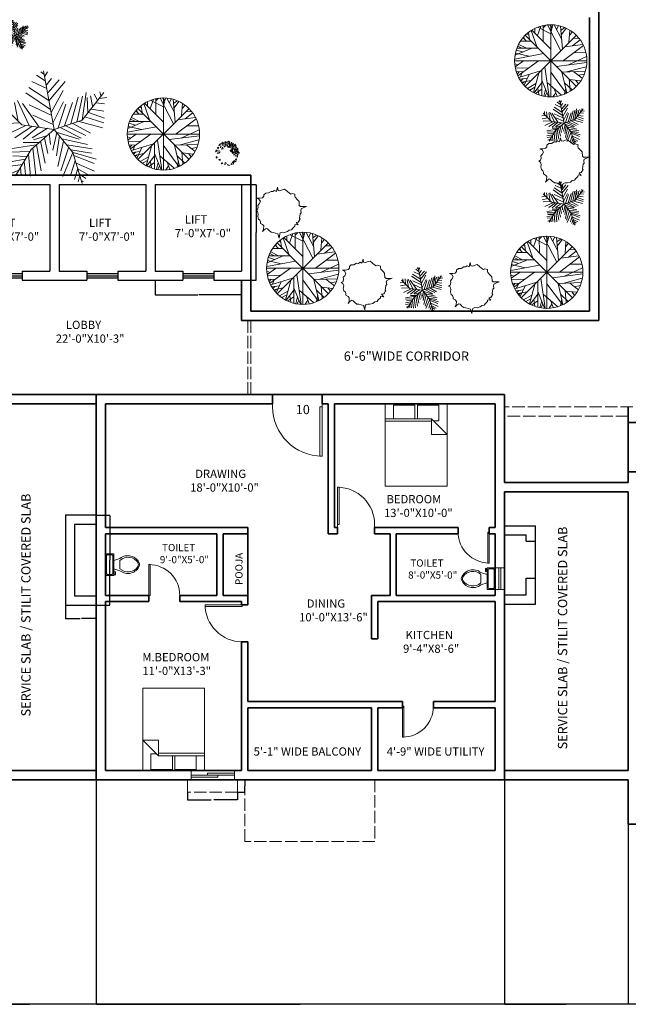
# Model space of a CAD drawing. Units: inches. Extents: x -69 to 2453, y 4803 to 7122.
# Tile 5 of 9: x 1203 to 1794, y 4803 to 5759. Entities that reach past the tile are written whole.
import ezdxf

# ---------------------------------------------------------------- set-up
doc = ezdxf.new("R2010")
doc.units = ezdxf.units.IN
doc.linetypes.add('ACAD_ISO02W100', pattern=[15, 12, -3])
for name, color, linetype, lineweight in [('A-ANNO-DIMS', 2, 'Continuous', 18), ('A-ANNO-IDEN', 2, 'Continuous', 18), ('A-AREA-IDEN', 7, 'Continuous', 18), ('A-DOOR', 3, 'Continuous', 18), ('A-FLOR-EVTR', 4, 'Continuous', 25), ('A-FLOR-FIXT', 9, 'Continuous', 18), ('A-FLOR-OVHD', 8, 'ACAD_ISO02W100', 13), ('A-FURN', 8, 'Continuous', 18), ('A-GLAZ', 244, 'Continuous', 18), ('A-WALL', 7, 'Continuous', 35), ('A-WALL-SRVC', 7, 'Continuous', 30), ('L-PLNT', 94, 'Continuous', 13)]:
    doc.layers.add(name, color=color, linetype=linetype, lineweight=lineweight)
doc.styles.get("Standard").update_dxf_attribs({"font": 'arial.ttf'})
doc.dimstyles.get("Standard").update_dxf_attribs({"dimtxt": 0.18, "dimasz": 0.18, "dimexe": 0.18, "dimexo": 0.0625, "dimgap": 0.09, "dimtad": 0, "dimtih": 1, "dimtoh": 1, "dimdec": 4, "dimzin": 0, "dimdsep": 46, "dimtxsty": 'Standard', "dimcen": 0.09, "dimadec": 0, "dimazin": 0, "dimtfac": 1, "dimtdec": 4, "dimtofl": 0, "dimtmove": 0, "dimatfit": 3, "dimfxl": 1, "dimtolj": 1, "dimtzin": 0, "dimarcsym": 0})

# ---------------------------------------------------------------- blocks, each defined once
blk = doc.blocks.new('*U6')
for p, q in [((-40, 0), (-40, 6)), ((0, 0), (0, 6))]:
    blk.add_line(p, q)
blk.add_lwpolyline([(0, 0), (0, -40), (-1.75, -40), (-1.75, 0)], close=True)
blk.add_arc((0, 0), 40, 180, 270)
blk = doc.blocks.new('*U17')
for p, q in [((0, 0), (0, 6)), ((40, 0), (40, 6))]:
    blk.add_line(p, q)
blk.add_lwpolyline([(0, 0), (0, -40), (1.75, -40), (1.75, 0)], close=True)
blk.add_arc((0, 0), 40, 270, 0)
blk = doc.blocks.new('*U5')
for p, q in [((0, 0), (0, -6)), ((40, 0), (40, -6))]:
    blk.add_line(p, q)
blk.add_lwpolyline([(0, 0), (0, 40), (1.75, 40), (1.75, 0)], close=True)
blk.add_arc((0, 0), 40, 0, 90)
blk = doc.blocks.new('*U3')
for p, q in [((0, 0), (0, 6)), ((40, 0), (40, 6))]:
    blk.add_line(p, q)
blk.add_lwpolyline([(0, 0), (0, -40), (1.75, -40), (1.75, 0)], close=True)
blk.add_arc((0, 0), 40, 270, 360)
blk = doc.blocks.new('*U22')
for p, q in [((0, 0), (0, -6)), ((40, 0), (40, -6))]:
    blk.add_line(p, q)
blk.add_lwpolyline([(0, 0), (0, 40), (1.75, 40), (1.75, 0)], close=True)
blk.add_arc((0, 0), 40, 0, 90)
blk = doc.blocks.new('*U29')
blk.add_lwpolyline([(-4.577, 66.508), (-7.629, 55.26), (-12.588, 57.705), (-17.165, 54.771), (-22.124, 55.26), (-29.372, 50.859), (-36.619, 50.37), (-41.578, 45.968), (-41.578, 42.056), (-45.393, 37.655), (-52.259, 36.677), (-60.651, 36.677), (-54.929, 33.743), (-51.115, 27.385), (-54.548, 21.028), (-58.362, 17.116), (-57.599, 11.248), (-58.744, 5.379), (-63.703, 2.445), (-59.125, 0), (-56.837, -6.846), (-58.362, -13.204), (-56.455, -20.539), (-52.259, -23.473), (-51.115, -27.386), (-51.115, -32.276), (-45.011, -35.21), (-41.96, -39.122), (-42.723, -47.925), (-45.393, -54.282), (-40.434, -49.392), (-35.475, -45.969), (-31.66, -46.947), (-27.083, -51.837), (-21.361, -56.238), (-16.021, -56.727), (-3.433, -60.151), (0, -71.887), (1.526, -60.151), (3.052, -58.194), (8.392, -56.238), (14.114, -56.727), (22.506, -54.282), (27.465, -50.37), (33.95, -49.392), (37.002, -44.991), (42.723, -39.611), (43.105, -35.699), (45.012, -34.721), (51.878, -36.188), (46.157, -29.342), (51.878, -28.364), (53.785, -25.919), (56.074, -21.517), (57.6, -20.539), (55.693, -18.094), (57.219, -5.868), (59.889, -2.934), (58.744, 3.423), (60.27, 7.824), (67.137, 11.248), (74.766, 14.182), (67.899, 13.693), (58.363, 13.693), (54.93, 16.627), (54.167, 27.874), (50.353, 32.276), (43.868, 39.122), (42.723, 42.545), (43.105, 47.436), (35.476, 49.881), (31.661, 47.925), (27.084, 50.859), (14.496, 61.128), (9.155, 59.661), (2.289, 56.727), (-3.051, 57.705)], close=True)
blk = doc.blocks.new('*U25')
for p, q in [((-8.737, 47.138), (-17.069, 52.711)), ((-10.186, 53.64), (-13.084, 55.962)), ((0, 0), (-10.5, 57)), ((-9.099, 51.782), (-6.563, 55.962)), ((-7.65, 43.423), (-2.578, 49.46)), ((-5.839, 35.992), (4.667, 48.067)), ((-5.114, 28.097), (-24.676, 40.636)), ((-7.288, 39.707), (-21.778, 46.673)), ((-5.114, 27.632), (10.463, 46.673)), ((-48.585, 21.131), (-49.309, 29.026)), ((-3.665, 19.273), (-27.574, 35.527)), ((-2.941, 16.486), (8.652, 37.85)), ((16.259, 5.805), (23.142, 31.348)), ((22.055, 7.198), (27.489, 32.277)), ((27, 9), (48, 36)), ((27.127, 9.056), (31.112, 35.992)), ((31.836, 30.883), (32.561, 16.486)), ((35.096, 32.741), (37.27, 22.524)), ((38.719, 34.134), (41.979, 28.561)), ((43.791, 29.954), (51.036, 30.883)), ((44.153, 36.456), (45.239, 32.741)), ((-47.498, 19.737), (-55.83, 18.344)), ((-31.5, 4.5), (-52.5, 25.5)), ((-43.513, 28.561), (-42.427, 15.558)), ((-38.442, 26.239), (-34.819, 7.663)), ((-35.544, 28.097), (-24.314, 3.947)), ((-14.533, 2.09), (-30.834, 25.31)), ((-24.314, 23.917), (-2.941, 13.7)), ((-1.129, 6.734), (9.014, 26.704)), ((3.942, 1.625), (11.187, 24.381)), ((10.101, 3.483), (17.708, 26.239)), ((36.183, 19.737), (48.137, 17.88)), ((40.53, 25.775), (48.862, 24.846)), ((-40.615, 13.7), (-55.105, 10.913)), ((-20.691, 13.7), (-1.129, 4.876)), ((29.662, 12.307), (48.137, 6.269)), ((33.285, 16.486), (48.862, 10.913)), ((-33.37, 6.269), (-52.207, 5.34)), ((-28.299, 3.483), (-47.86, -5.805)), ((-21.416, 3.018), (-38.079, -8.128)), ((0, 0), (-31.5, 4.5)), ((-15.982, 2.09), (-30.11, -9.521)), ((0, 0), (-22.5, -19.5)), ((-6.563, 1.161), (-21.416, -8.128)), ((0, 0), (27, 9)), ((0, 0), (18, -22.5)), ((6.478, 1.625), (26.04, -8.592)), ((11.187, 3.483), (30.749, -5.805)), ((18.07, 5.805), (35.096, -3.483)), ((24.229, 7.663), (46.688, 1.625)), ((-6.563, -5.805), (-19.967, -9.985)), ((-9.461, -8.592), (-6.201, -23.453)), ((-4.752, -3.483), (-3.665, -14.629)), ((2.493, -3.019), (-1.491, -20.202)), ((1.769, -2.555), (24.229, -9.521)), ((5.029, -6.27), (2.131, -25.775)), ((7.565, -9.056), (32.198, -14.629)), ((-17.431, -15.094), (-42.789, -18.809)), ((-15.257, -12.772), (-30.11, -12.772)), ((-20.691, -18.345), (-17.793, -44.352)), ((-17.069, -15.094), (-12.721, -40.172)), ((-13.446, -11.378), (-8.737, -32.741)), ((9.014, -11.378), (3.58, -35.992)), ((14.085, -16.951), (6.478, -40.172)), ((12.274, -15.094), (36.907, -18.809)), ((-24.314, -21.596), (-42.427, -22.06)), ((-26.849, -26.24), (-40.253, -25.775)), ((-22.5, -19.5), (-37.5, -45)), ((-25.038, -23.918), (-22.865, -45.281)), ((18.07, -22.524), (8.289, -45.745)), ((16.259, -19.738), (36.183, -22.989)), ((18, -22.5), (27, -52.5)), ((18.433, -22.524), (40.53, -29.026)), ((19.157, -25.311), (38.719, -33.206)), ((-28.299, -29.026), (-42.789, -31.348)), ((-30.834, -34.135), (-42.427, -35.528)), ((-32.646, -36.921), (-31.921, -44.352)), ((-29.023, -30.884), (-27.936, -43.887)), ((20.244, -30.419), (15.897, -44.816)), ((22.78, -37.85), (19.519, -48.532)), ((21.331, -32.741), (39.081, -40.636)), ((-34.457, -39.708), (-40.978, -42.494)), ((22.78, -38.314), (34.372, -44.816)), ((24.591, -45.745), (23.142, -50.854)), ((24.591, -43.423), (30.749, -47.603)), ((26.764, -49.925), (28.213, -50.854))]:
    blk.add_line(p, q)
blk = doc.blocks.new('*U28')
for p, q in [((-32.6092, 50.4264), (-23.2782, 23.5674)), ((-31.2008, 51.1035), (-0.2149, 20.1818)), ((-26.4472, 46.5894), (-26.2712, 53.8116)), ((-22.0458, 42.0753), (-16.5881, 57.6486)), ((-21.1656, 55.8436), (-0.0388, 45.0094)), ((-12.5388, 54.9406), (-7.9613, 59.4546)), ((-12.3627, 32.1443), (-12.5388, 58.7776)), ((-5.3205, 59.6806), (16.5105, 16.7963)), ((2.426, 54.9406), (-1.4472, 59.9056)), ((0, 59.9996), (0, -60)), ((0.4894, 48.6208), (3.6584, 59.6806)), ((18.2711, 35.5298), (5.419, 59.6806)), ((9.8203, 51.5549), (12.8133, 58.5516)), ((19.6795, 19.5047), (16.3344, 57.6486)), ((17.0387, 51.1035), (23.2006, 55.1666)), ((17.7429, 43.6552), (25.4894, 54.2636)), ((31.6513, 50.8778), (30.2429, 30.5643)), ((-49.8627, 32.8214), (-32.7853, 32.8214)), ((-45.8134, 38.2383), (-40.5318, 33.0471)), ((-43.8768, 36.4326), (-44.405, 40.2696)), ((42, 42), (-42, -42)), ((42, -42), (-42, 42)), ((-40.1797, 44.558), (-36.4825, 43.2038)), ((-37.0107, 47.0408), (-35.25, 35.5298)), ((31.1232, 42.5267), (35.8767, 48.1693)), ((36.2288, 25.1474), (48.9049, 35.0784)), ((37.1091, 37.1098), (46.6161, 37.5612)), ((-32.2571, 20.6333), (-59.1937, 9.348)), ((-57.081, 17.9248), (-47.0458, 14.7649)), ((-56.0247, 20.859), (-20.8134, 20.859)), ((-54.7923, 24.4702), (-47.75, 21.0847)), ((-53.2078, 27.4044), (-40.1797, 20.859)), ((54.3626, 25.3731), (20.9119, 0.3198)), ((23.3767, 23.3417), (53.3063, 27.4044)), ((-59.7219, 2.8025), (-12.0106, 12.0565)), ((-58.6656, 12.7336), (-35.9543, 7.5424)), ((-54.6162, -24.7335), (-20.2853, 0.0941)), ((29.3626, -6.6771), (59.4682, 7.091)), ((38.5175, 13.4107), (58.2359, 13.6364)), ((-60, 0), (60, 0)), ((-59.7219, -4.8714), (-54.2641, -6.6771)), ((-45.2853, -0.1316), (-59.0177, -10.0627)), ((-58.4895, -12.3197), (-36.4825, -11.6426)), ((-14.8275, -15.0282), (-14.6515, -57.6865)), ((-10.074, -10.0627), (-2.5036, -59.7178)), ((9.2922, -9.1598), (59.6443, -2.8401)), ((26.3697, -18.4138), (58.9401, -9.8369)), ((-57.081, -18.4138), (-45.2853, -17.9624)), ((-52.6797, -18.188), (-55.4966, -22.0251)), ((-53.2078, -27.442), (-16.7641, -16.6081)), ((-38.9472, -29.0219), (-51.4472, -30.6018)), ((-47.2219, -19.3166), (-50.2148, -26.3135)), ((-46.5177, -30.1504), (-49.5106, -33.536)), ((-32.4331, -32.4075), (-48.1021, -35.5674)), ((-35.9543, -22.4765), (-44.0529, -40.5329)), ((-19.9331, -20.2194), (-28.5599, -52.721)), ((-14.6515, -32.1818), (-3.912, -59.4922)), ((-0.0388, -19.0909), (25.8415, -53.8495)), ((18.6232, -18.6394), (26.7218, -53.3981)), ((18.7992, -18.6394), (57.3556, -17.2853)), ((30.419, -30.1504), (32.3556, -50.0125)), ((31.4753, -31.279), (49.6091, -33.3103)), ((38.1654, -18.188), (52.426, -29.0219)), ((41.5105, -32.6332), (46.088, -38.0501)), ((45.9119, -24.0564), (55.595, -22.2508)), ((-43.7008, -34.6645), (-46.6937, -37.373)), ((-24.6867, -37.8244), (-38.7712, -45.7241)), ((-26.2712, -43.9185), (-34.7219, -48.6583)), ((-14.6515, -36.2445), (-27.6797, -52.9467)), ((-14.6515, -47.3041), (-25.0388, -54.3009)), ((-21.5177, -45.4984), (-19.9331, -56.1065)), ((-8.4895, -47.5298), (-11.4825, -58.5893)), ((-6.2008, -36.2445), (17.919, -57.0094)), ((5.9471, -46.6269), (10.5246, -58.5893)), ((22.8485, -36.4702), (35.3485, -48.4326)), ((24.7852, -44.8213), (23.0246, -54.978)), ((-6.3768, -52.721), (-9.3698, -58.815)), ((8.4119, -53.1724), (3.8344, -59.4922))]:
    blk.add_line(p, q)
blk.add_circle((0, 0), 60)
blk = doc.blocks.new('*U27')
for points in [[(-5.78, 9.75), (-7.54, 9.23), (-8.01, 7.5), (-6.26, 8.45)], [(-4.43, 11.05), (-5.18, 10.36), (-3.96, 9.49), (-2.07, 10.36)], [(-2, 11.66), (-1.6, 10.62), (-0.52, 10.1), (-0.18, 10.62), (-0.79, 10.96)], [(1.24, 12), (0.56, 11.31), (0.76, 10.01), (2.52, 11.05)], [(2.59, 9.93), (1.84, 9.75), (1.64, 9.23), (2.32, 9.41)], [(4.14, 11.14), (3.6, 10.01), (4, 9.23), (5.22, 8.71), (6.3, 9.41), (5.08, 10.19), (4.61, 10.01)], [(-11.32, 1.79), (-9.83, 2.31), (-9.63, 3.44), (-10.44, 3.52)], [(-8.21, 0.41), (-9.43, 0.32), (-9.83, 0.84)], [(-8.14, 6.03), (-9.36, 5.95), (-9.02, 4.73)], [(-8.21, 3.09), (-8.48, 2.31), (-7.87, 2.57)], [(-7, 1.79), (-7.94, 1.53), (-7.47, 0.49)], [(-5.78, 6.81), (-6.66, 6.21), (-6.52, 5.69)], [(-4.57, 6.38), (-5.45, 4.47), (-3.89, 4.82)], [(-4.84, 8.63), (-3.83, 7.85), (-4.03, 8.97)], [(-2.88, 7.5), (-3.15, 6.64), (-2.27, 6.72)], [(-1.94, 9.49), (-2.48, 8.97), (-2.27, 8.54), (-1.8, 9.06)], [(0.02, 9.06), (-1.33, 8.54), (-1.73, 7.16), (0.29, 7.76)], [(0.76, 7.16), (0.09, 6.46), (1.1, 5.95)], [(1.37, 8.54), (3.13, 8.8), (3.8, 7.85), (1.91, 7.76)], [(1.71, 6.29), (1.71, 7.07), (2.65, 7.5), (2.11, 6.9)], [(2.52, 6.81), (2.52, 5.86), (4.41, 5.17), (4.61, 6.72)], [(3.53, 1.88), (2.86, 3.52), (3.8, 3.52)], [(4.41, 4.56), (4.27, 3.7), (5.49, 3.26)], [(4.27, 2.74), (5.29, 2.66), (4.41, 1.27)], [(4.61, 8.28), (4.54, 7.76), (4.95, 7.59), (4.95, 8.28)], [(5.83, 1.53), (5.02, 0.41), (5.49, -0.02), (6.5, 0.41)], [(5.49, 5.51), (5.42, 4.82), (6.16, 5.08)], [(6.43, 7.94), (5.49, 7.68), (5.56, 6.21), (6.5, 6.64)], [(7.51, 1.71), (6.91, 1.27), (6.23, 2.14)], [(8.12, 4.99), (7.11, 4.65), (6.5, 4.13), (7.38, 3.09), (8.12, 3.52), (7.65, 3.87)], [(7.45, 9.32), (7.11, 7.94), (8.52, 7.94)], [(7.85, 6.81), (7.18, 6.21), (9, 5.51), (9.33, 6.38)], [(8.12, 0.75), (7.51, 0.15), (8.93, -0.28), (9.13, 0.49)], [(8.19, 2.57), (7.92, 2.05), (8.66, 1.53)], [(8.73, 4.73), (8.19, 4.56), (8.39, 3.87), (8.59, 4.04)], [(10.28, 5.17), (9.2, 4.04), (9, 2.31), (10.48, 0.49), (11.76, 0.41), (10.35, 2.48), (9.33, 2.4), (10.28, 2.83)], [(-10.03, -2.71), (-10.64, -3.31), (-10.44, -4.44), (-9.9, -3.49)], [(-8.28, -5.73), (-6.79, -5.3), (-7, -6.51)], [(-4.84, -8.85), (-4.43, -9.45), (-5.99, -9.8)], [(-2.34, -9.2), (-1.26, -8.5), (-0.99, -9.54)], [(4.07, -9.45), (3.53, -9.97), (4.07, -10.58), (4.61, -9.89)], [(5.29, -7.98), (4.61, -8.16), (5.02, -8.94)], [(6.03, -9.45), (5.42, -9.97), (6.16, -10.15)], [(6.1, -8.94), (6.16, -7.21), (6.91, -6.69), (7.24, -7.38)], [(7.78, -0.8), (6.43, -1.5), (6.43, -0.72)], [(8.32, -1.75), (7.98, -2.53), (7.58, -2.1)], [(8.05, -8.07), (8.59, -7.12), (7.92, -7.55)], [(9.33, -5.13), (8.46, -6.25), (7.98, -5.22)], [(9.33, -1.75), (9.54, -3.74), (10.14, -2.53)], [(10.08, -0.63), (9.74, -1.32), (10.48, -0.89)], [(-2.54, -10.06), (-3.02, -10.23), (-1.8, -10.67)], [(0.22, -10.58), (0.83, -11.27), (2.59, -11.36)]]:
    blk.add_lwpolyline(points, close=True)
blk = doc.blocks.new('Bed - Queen')
for p, q in [((0, -80.00003), (0, 0)), ((0, 0), (59.99999, 0)), ((59.99999, 0), (59.99999, -80.00003)), ((7.99999, -1.2), (28.79998, -1.2)), ((7.99999, -14.4), (7.99999, -1.2)), ((28.79998, -1.2), (28.79998, -14.4)), ((31.19999, -1.2), (51.99999, -1.2)), ((31.19999, -14.4), (31.19999, -1.2)), ((51.99999, -1.2), (51.99999, -16.4)), ((0, -14.4), (44.8, -14.4)), ((44.8, -16.8), (0, -16.8)), ((59.99999, -29.6), (44.8, -14.4)), ((44.8, -14.4), (44.8, -29.6)), ((51.99999, -16.4), (46.79936, -16.4)), ((44.8, -29.6), (59.99999, -29.6)), ((59.99999, -80.00003), (0, -80.00003))]:
    blk.add_line(p, q)
blk = doc.blocks.new('*U33')
for p, q in [((-10, -8.5), (-8, -8.5)), ((-10, -9.5), (-10, -8.5)), ((-7, -9.5), (-10, -9.5)), ((-8, -8.5), (-8, -8)), ((-7, -8), (-7, -9.5)), ((-4, -8), (-6, -14)), ((4, -8), (6, -14)), ((9.5, -6), (9.5, -2)), ((4, -14), (-4, -14))]:
    blk.add_line(p, q)
blk.add_lwpolyline([(10.5, -8), (10.5, 0), (-10.5, 0), (-10.5, -8)], close=True)
for points in [[(-9.5, -2), (-9.5, -6)], [(8.5, -1), (-8.5, -1)], [(-8.5, -7), (8.5, -7)]]:
    blk.add_lwpolyline(points)
for centre, radius, start, end in [((-8.62, -1.88), 0.884, 81.8699, 188.1301), ((-8.62, -6.12), 0.884, 171.8699, 278.1301), ((8.62, -1.88), 0.884, 351.8699, 98.1301), ((8.62, -6.12), 0.884, 261.8699, 8.1301), ((3.52, -21.58), 12.17, 141.46911, 247.97143), ((4.2, -21.82), 11.33, 136.36773, 238.94682), ((-3.52, -21.58), 12.17, 292.02843, 38.53071), ((-4.2, -21.82), 11.33, 301.05301, 43.63209), ((0, -27.88), 4, 245.73182, 294.26817), ((0, -29), 4, 254.86053, 285.13947)]:
    blk.add_arc(centre, radius, start, end)
blk = doc.blocks.new('WINDOW-VENT-21IN')
for p, q in [((0, 5.5), (21, 5.5)), ((0, 3.5), (21, 3.5))]:
    blk.add_line(p, q)
blk.add_lwpolyline([(0, 9), (21, 9), (21, 0), (0, 0)], close=True)
blk = doc.blocks.new('WINDOW-SLIDING-42IN')
for p, q in [((2.5, 42), (2.5, 16)), ((4.5, 42), (4.5, 0)), ((4.5, 26), (6.5, 26)), ((6.5, 26), (6.5, 0)), ((4.5, 16), (2.5, 16))]:
    blk.add_line(p, q)
blk.add_lwpolyline([(0, 42), (9, 42), (9, 0), (0, 0)], close=True)
blk = doc.blocks.new('SUNSHADE-48IN')
for p, q in [((0, 0), (0, 12)), ((48.4, 12), (48.4, 0)), ((48.4, 0), (0, 0))]:
    blk.add_line(p, q)
blk = doc.blocks.new('SERVICE-BAY-87IN')
for p, q in [((30, 87.24), (0, 87.24)), ((0, 87.24), (0, 0)), ((30, 78.24), (9, 78.24)), ((9, 78.24), (9, 9)), ((0, 0), (30, 0)), ((9, 9), (30, 9))]:
    blk.add_line(p, q)
blk = doc.blocks.new('LIFT-PASSENGER-84IN')
for p, q in [((0, 93), (84, 93)), ((0, 93), (0, 9)), ((84, 93), (84, 9)), ((0, 9), (27, 9)), ((27, 9), (27, 0)), ((27, 6.5), (57, 6.5)), ((27, 4.5), (57, 4.5)), ((27, 2.5), (57, 2.5)), ((57, 9), (57, 0)), ((57, 9), (84, 9))]:
    blk.add_line(p, q)
blk = doc.blocks.new('*D55')
at = {"layer": 'A-ANNO-DIMS', "color": 0, "lineweight": -2, "transparency": 16777216}
for p, q in [((1365.97, 5008.65), (1365.97, 5001.28)), ((1366.15, 5001.46), (1388.91, 5001.46)), ((1414.19, 5001.46), (1391.43, 5001.46)), ((1414.37, 5008.65), (1414.37, 5001.28))]:
    blk.add_line(p, q, dxfattribs=at)
at = {"layer": 'A-ANNO-DIMS', "color": 0, "transparency": 16777216}
for points in [[(1366.15, 5001.49), (1366.15, 5001.43), (1365.97, 5001.46)], [(1414.19, 5001.49), (1414.19, 5001.43), (1414.37, 5001.46)]]:
    blk.add_solid(points, dxfattribs=at)
at = {"layer": 'Defpoints', "color": 0, "transparency": 16777216}
for p in [(1365.97, 5008.72), (1414.37, 5008.72), (1414.37, 5001.46)]:
    blk.add_point(p, dxfattribs=at)
at = {"layer": 'A-ANNO-DIMS', "color": 0, "transparency": 16777216, "insert": (1390.17, 5001.46), "char_height": 0.18, "attachment_point": 5}
blk.add_mtext('\\A1;SUNSHADE 48 TYP.', dxfattribs=at)
blk = doc.blocks.new('*D56')
at = {"layer": 'A-ANNO-DIMS', "color": 0, "lineweight": -2, "transparency": 16777216}
for p, q in [((1414.43, 5020.72), (1421.81, 5020.72)), ((1421.63, 5020.54), (1421.63, 5014.9)), ((1421.63, 5008.9), (1421.63, 5014.53)), ((1414.43, 5008.72), (1421.81, 5008.72))]:
    blk.add_line(p, q, dxfattribs=at)
at = {"layer": 'A-ANNO-DIMS', "color": 0, "transparency": 16777216}
for points in [[(1421.6, 5020.54), (1421.66, 5020.54), (1421.63, 5020.72)], [(1421.6, 5008.9), (1421.66, 5008.9), (1421.63, 5008.72)]]:
    blk.add_solid(points, dxfattribs=at)
at = {"layer": 'Defpoints', "color": 0, "transparency": 16777216}
for p in [(1414.37, 5020.72), (1421.63, 5020.72), (1414.37, 5008.72)]:
    blk.add_point(p, dxfattribs=at)
at = {"layer": 'A-ANNO-DIMS', "color": 0, "transparency": 16777216, "insert": (1421.63, 5014.72), "char_height": 0.18, "attachment_point": 5}
blk.add_mtext('\\A1;12 TYP.', dxfattribs=at)
blk = doc.blocks.new('*D71')
at = {"layer": 'A-ANNO-DIMS', "color": 0, "lineweight": -2, "transparency": 16777216}
for p, q in [((1418.57, 5598.72), (1432.64, 5598.72)), ((1432.46, 5598.54), (1432.46, 5552.4)), ((1432.46, 5505.9), (1432.46, 5552.03)), ((1418.57, 5505.72), (1432.64, 5505.72))]:
    blk.add_line(p, q, dxfattribs=at)
at = {"layer": 'A-ANNO-DIMS', "color": 0, "transparency": 16777216}
for points in [[(1432.43, 5598.54), (1432.49, 5598.54), (1432.46, 5598.72)], [(1432.43, 5505.9), (1432.49, 5505.9), (1432.46, 5505.72)]]:
    blk.add_solid(points, dxfattribs=at)
at = {"layer": 'Defpoints', "color": 0, "transparency": 16777216}
for p in [(1418.51, 5598.72), (1432.46, 5598.72), (1418.51, 5505.72)]:
    blk.add_point(p, dxfattribs=at)
at = {"layer": 'A-ANNO-DIMS', "color": 0, "transparency": 16777216, "insert": (1432.46, 5552.22), "char_height": 0.18, "attachment_point": 5}
blk.add_mtext('\\A1;PASSENGER LIFT 93 TYP.', dxfattribs=at)
blk = doc.blocks.new('*D72')
at = {"layer": 'A-ANNO-DIMS', "color": 0, "lineweight": -2, "transparency": 16777216}
for p, q in [((1334.51, 5505.65), (1334.51, 5491.59)), ((1418.51, 5505.65), (1418.51, 5491.59)), ((1334.69, 5491.77), (1375.98, 5491.77)), ((1418.33, 5491.77), (1377.04, 5491.77))]:
    blk.add_line(p, q, dxfattribs=at)
at = {"layer": 'A-ANNO-DIMS', "color": 0, "transparency": 16777216}
for points in [[(1334.69, 5491.8), (1334.69, 5491.74), (1334.51, 5491.77)], [(1418.33, 5491.8), (1418.33, 5491.74), (1418.51, 5491.77)]]:
    blk.add_solid(points, dxfattribs=at)
at = {"layer": 'Defpoints', "color": 0, "transparency": 16777216}
for p in [(1334.51, 5505.72), (1418.51, 5505.72), (1418.51, 5491.77)]:
    blk.add_point(p, dxfattribs=at)
at = {"layer": 'A-ANNO-DIMS', "color": 0, "transparency": 16777216, "insert": (1376.51, 5491.77), "char_height": 0.18, "attachment_point": 5}
blk.add_mtext('\\A1;84 TYP.', dxfattribs=at)
blk = doc.blocks.new('*D77')
at = {"layer": 'A-ANNO-DIMS', "color": 0, "lineweight": -2, "transparency": 16777216}
for p, q in [((1277.57, 5277.65), (1290.78, 5277.65)), ((1290.6, 5277.47), (1290.6, 5234.21)), ((1290.6, 5190.59), (1290.6, 5233.84)), ((1277.57, 5190.41), (1290.78, 5190.41))]:
    blk.add_line(p, q, dxfattribs=at)
at = {"layer": 'A-ANNO-DIMS', "color": 0, "transparency": 16777216}
for points in [[(1290.57, 5277.47), (1290.63, 5277.47), (1290.6, 5277.65)], [(1290.57, 5190.59), (1290.63, 5190.59), (1290.6, 5190.41)]]:
    blk.add_solid(points, dxfattribs=at)
at = {"layer": 'Defpoints', "color": 0, "transparency": 16777216}
for p in [(1277.51, 5277.65), (1290.6, 5277.65), (1277.51, 5190.41)]:
    blk.add_point(p, dxfattribs=at)
at = {"layer": 'A-ANNO-DIMS', "color": 0, "transparency": 16777216, "insert": (1290.6, 5234.03), "char_height": 0.18, "attachment_point": 5}
blk.add_mtext('\\A1;SERVICE BAY 87 TYP.', dxfattribs=at)
blk = doc.blocks.new('*D78')
at = {"layer": 'A-ANNO-DIMS', "color": 0, "lineweight": -2, "transparency": 16777216}
for p, q in [((1247.51, 5190.34), (1247.51, 5177.14)), ((1277.51, 5190.34), (1277.51, 5177.14)), ((1247.69, 5177.32), (1261.98, 5177.32)), ((1277.33, 5177.32), (1263.04, 5177.32))]:
    blk.add_line(p, q, dxfattribs=at)
at = {"layer": 'A-ANNO-DIMS', "color": 0, "transparency": 16777216}
for points in [[(1247.69, 5177.35), (1247.69, 5177.29), (1247.51, 5177.32)], [(1277.33, 5177.35), (1277.33, 5177.29), (1277.51, 5177.32)]]:
    blk.add_solid(points, dxfattribs=at)
at = {"layer": 'Defpoints', "color": 0, "transparency": 16777216}
for p in [(1247.51, 5190.41), (1277.51, 5190.41), (1277.51, 5177.32)]:
    blk.add_point(p, dxfattribs=at)
at = {"layer": 'A-ANNO-DIMS', "color": 0, "transparency": 16777216, "insert": (1262.51, 5177.32), "char_height": 0.18, "attachment_point": 5}
blk.add_mtext('\\A1;30 TYP.', dxfattribs=at)
blk = doc.blocks.new('*D84')
at = {"layer": 'A-ANNO-DIMS', "color": 0, "lineweight": -2, "transparency": 16777216}
for p, q in [((1148.51, 5020.65), (1148.51, 4802.79)), ((1277.51, 5020.65), (1277.51, 4802.79)), ((1148.69, 4802.97), (1212.73, 4802.97)), ((1277.33, 4802.97), (1213.29, 4802.97))]:
    blk.add_line(p, q, dxfattribs=at)
at = {"layer": 'A-ANNO-DIMS', "color": 0, "transparency": 16777216}
for points in [[(1148.69, 4803), (1148.69, 4802.94), (1148.51, 4802.97)], [(1277.33, 4803), (1277.33, 4802.94), (1277.51, 4802.97)]]:
    blk.add_solid(points, dxfattribs=at)
at = {"layer": 'Defpoints', "color": 0, "transparency": 16777216}
for p in [(1148.51, 5020.72), (1277.51, 5020.72), (1277.51, 4802.97)]:
    blk.add_point(p, dxfattribs=at)
at = {"layer": 'A-ANNO-DIMS', "color": 0, "transparency": 16777216, "insert": (1213.01, 4802.97), "char_height": 0.18, "attachment_point": 5}
blk.add_mtext('\\A1;129', dxfattribs=at)
blk = doc.blocks.new('*D85')
at = {"layer": 'A-ANNO-DIMS', "color": 0, "lineweight": -2, "transparency": 16777216}
for p, q in [((1277.51, 5020.65), (1277.51, 4802.79)), ((1673.51, 5020.65), (1673.51, 4802.79)), ((1277.69, 4802.97), (1475.22, 4802.97)), ((1673.33, 4802.97), (1475.8, 4802.97))]:
    blk.add_line(p, q, dxfattribs=at)
at = {"layer": 'A-ANNO-DIMS', "color": 0, "transparency": 16777216}
for points in [[(1277.69, 4803), (1277.69, 4802.94), (1277.51, 4802.97)], [(1673.33, 4803), (1673.33, 4802.94), (1673.51, 4802.97)]]:
    blk.add_solid(points, dxfattribs=at)
at = {"layer": 'Defpoints', "color": 0, "transparency": 16777216}
for p in [(1277.51, 5020.72), (1673.51, 5020.72), (1673.51, 4802.97)]:
    blk.add_point(p, dxfattribs=at)
at = {"layer": 'A-ANNO-DIMS', "color": 0, "transparency": 16777216, "insert": (1475.51, 4802.97), "char_height": 0.18, "attachment_point": 5}
blk.add_mtext('\\A1;396', dxfattribs=at)
blk = doc.blocks.new('*D86')
at = {"layer": 'A-ANNO-DIMS', "color": 0, "lineweight": -2, "transparency": 16777216}
for p, q in [((1673.51, 5020.65), (1673.51, 4802.79)), ((1793.51, 5020.65), (1793.51, 4802.79)), ((1673.69, 4802.97), (1733.23, 4802.97)), ((1793.33, 4802.97), (1733.79, 4802.97))]:
    blk.add_line(p, q, dxfattribs=at)
at = {"layer": 'A-ANNO-DIMS', "color": 0, "transparency": 16777216}
for points in [[(1673.69, 4803), (1673.69, 4802.94), (1673.51, 4802.97)], [(1793.33, 4803), (1793.33, 4802.94), (1793.51, 4802.97)]]:
    blk.add_solid(points, dxfattribs=at)
at = {"layer": 'Defpoints', "color": 0, "transparency": 16777216}
for p in [(1673.51, 5020.72), (1793.51, 5020.72), (1793.51, 4802.97)]:
    blk.add_point(p, dxfattribs=at)
at = {"layer": 'A-ANNO-DIMS', "color": 0, "transparency": 16777216, "insert": (1733.51, 4802.97), "char_height": 0.18, "attachment_point": 5}
blk.add_mtext('\\A1;120', dxfattribs=at)
blk = doc.blocks.new('*D95')
at = {"layer": 'A-ANNO-DIMS', "color": 0, "lineweight": -2, "transparency": 16777216}
for p, q in [((96.509262, 5020.652777), (96.509262, 4802.785277)), ((2286.509262, 4977.652777), (2286.509262, 4802.785277)), ((96.689262, 4802.965277), (1191.149262, 4802.965277)), ((2286.329262, 4802.965277), (1191.869262, 4802.965277))]:
    blk.add_line(p, q, dxfattribs=at)
at = {"layer": 'A-ANNO-DIMS', "color": 0, "transparency": 16777216}
for points in [[(96.689262, 4802.995277), (96.689262, 4802.935277), (96.509262, 4802.965277)], [(2286.329262, 4802.995277), (2286.329262, 4802.935277), (2286.509262, 4802.965277)]]:
    blk.add_solid(points, dxfattribs=at)
at = {"layer": 'Defpoints', "color": 0, "transparency": 16777216}
for p in [(96.509262, 5020.715277), (2286.509262, 4977.715277), (2286.509262, 4802.965277)]:
    blk.add_point(p, dxfattribs=at)
at = {"layer": 'A-ANNO-DIMS', "color": 0, "transparency": 16777216, "insert": (1191.509262, 4802.965277), "char_height": 0.18, "attachment_point": 5}
blk.add_mtext('\\A1;2190', dxfattribs=at)
blk = doc.blocks.new('*D105')
at = {"layer": 'A-ANNO-DIMS', "color": 0, "lineweight": -2, "transparency": 16777216}
for p, q in [((66.509262, 5170.610035), (66.509262, 4802.785277)), ((2316.509262, 5140.587945), (2316.509262, 4802.785277)), ((66.689262, 4802.965277), (1191.149262, 4802.965277)), ((2316.329262, 4802.965277), (1191.869262, 4802.965277))]:
    blk.add_line(p, q, dxfattribs=at)
at = {"layer": 'A-ANNO-DIMS', "color": 0, "transparency": 16777216}
for points in [[(66.689262, 4802.995277), (66.689262, 4802.935277), (66.509262, 4802.965277)], [(2316.329262, 4802.995277), (2316.329262, 4802.935277), (2316.509262, 4802.965277)]]:
    blk.add_solid(points, dxfattribs=at)
at = {"layer": 'Defpoints', "color": 0, "transparency": 16777216}
for p in [(66.509262, 5170.672535), (2316.509262, 5140.650445), (2316.509262, 4802.965277)]:
    blk.add_point(p, dxfattribs=at)
at = {"layer": 'A-ANNO-DIMS', "color": 0, "transparency": 16777216, "insert": (1191.509262, 4802.965277), "char_height": 0.18, "attachment_point": 5}
blk.add_mtext('\\A1;2250', dxfattribs=at)

msp = doc.modelspace()

# ---------------------------------------------------------------- linework, layer by layer
at = {"layer": 'A-FLOR-EVTR'}
for p, q in [((1205.51, 5505.72), (1268.51, 5505.72)), ((1298.51, 5505.72), (1361.51, 5505.72)), ((1391.51, 5505.72), (1418.51, 5505.72))]:
    msp.add_line(p, q, dxfattribs=at)
at = {"layer": 'A-FLOR-OVHD'}
for p, q in [((1424.51, 5466.72), (1424.51, 5394.72)), ((1427.51, 5466.72), (1427.51, 5394.72)), ((1843.01, 5382.72), (1673.51, 5382.72)), ((1793.51, 5373.72), (1673.51, 5373.72)), ((1421.76, 4960.72), (1421.76, 5020.72)), ((1547.6, 5020.72), (1547.6, 4960.72)), ((1547.6, 4960.72), (1421.76, 4960.72))]:
    msp.add_line(p, q, dxfattribs=at)
at = {"layer": 'A-WALL'}
for p, q in [((1765.01, 6087.72), (1765.01, 5466.72)), ((1756.01, 5760.72), (1756.01, 5475.72)), ((857.51, 5607.72), (1427.51, 5607.72)), ((1427.51, 5607.72), (1427.51, 5475.72)), ((1418.51, 5505.72), (1418.51, 5466.72)), ((1427.51, 5475.72), (1756.01, 5475.72)), ((1418.51, 5466.72), (1765.01, 5466.72)), ((752.51, 5394.72), (1673.51, 5394.72)), ((1277.51, 5394.72), (1277.51, 5020.72)), ((1448.51, 5385.72), (1448.51, 5394.72)), ((1496.51, 5385.72), (1496.51, 5394.72)), ((1673.51, 5394.72), (1673.51, 5309.33)), ((1148.51, 5385.72), (1277.51, 5385.72)), ((1286.51, 5385.72), (1286.51, 5265.72)), ((1286.51, 5385.72), (1448.51, 5385.72)), ((1496.51, 5385.72), (1502.51, 5385.72)), ((1502.51, 5385.72), (1502.51, 5259.72)), ((1508.51, 5385.72), (1508.51, 5265.72)), ((1508.51, 5385.72), (1664.51, 5385.72)), ((1664.51, 5385.72), (1664.51, 5265.72)), ((1793.51, 5382.72), (1793.51, 5309.33)), ((1802.51, 5367.72), (1793.51, 5367.72)), ((1802.51, 5319.72), (1793.51, 5319.72)), ((1673.51, 5309.33), (1793.51, 5309.33)), ((1673.51, 5300.33), (1793.51, 5300.33)), ((1673.51, 5300.33), (1673.51, 5020.72)), ((1793.51, 5300.33), (1793.51, 5029.72)), ((1286.51, 5265.72), (1424.51, 5265.72)), ((1286.51, 5259.72), (1394.51, 5259.72)), ((1286.51, 5259.72), (1286.51, 5199.72)), ((1394.51, 5259.72), (1394.51, 5199.72)), ((1400.51, 5259.72), (1400.51, 5199.72)), ((1400.51, 5259.72), (1424.51, 5259.72)), ((1424.51, 5265.72), (1424.51, 5190.72)), ((1502.51, 5259.72), (1511.51, 5259.72)), ((1508.51, 5265.72), (1511.51, 5265.72)), ((1511.51, 5265.72), (1511.51, 5259.72)), ((1547.51, 5265.72), (1547.51, 5259.72)), ((1547.51, 5265.72), (1628.51, 5265.72)), ((1547.51, 5259.72), (1562.51, 5259.72)), ((1562.51, 5259.72), (1562.51, 5199.72)), ((1568.51, 5259.72), (1568.51, 5199.72)), ((1568.51, 5259.72), (1628.51, 5259.72)), ((1628.51, 5265.72), (1628.51, 5259.72)), ((1658.51, 5265.72), (1658.51, 5259.72)), ((1658.51, 5265.72), (1664.51, 5265.72)), ((1658.51, 5259.72), (1664.51, 5259.72)), ((1664.51, 5259.72), (1664.51, 5199.72)), ((1286.51, 5199.72), (1328.51, 5199.72)), ((1286.51, 5193.72), (1328.51, 5193.72)), ((1286.51, 5193.72), (1286.51, 5029.72)), ((1328.51, 5199.72), (1328.51, 5193.72)), ((1358.51, 5199.72), (1358.51, 5193.72)), ((1358.51, 5199.72), (1394.51, 5199.72)), ((1358.51, 5193.72), (1418.51, 5193.72)), ((1400.51, 5199.72), (1424.51, 5199.72)), ((1418.51, 5193.72), (1418.51, 5190.72)), ((1544.51, 5199.72), (1562.51, 5199.72)), ((1544.51, 5199.72), (1544.51, 5157.72)), ((1550.51, 5193.72), (1664.51, 5193.72)), ((1550.51, 5193.72), (1550.51, 5157.72)), ((1568.51, 5199.72), (1664.51, 5199.72)), ((1664.51, 5193.72), (1664.51, 5096.72)), ((1418.51, 5190.72), (1424.51, 5190.72)), ((1418.51, 5154.72), (1424.51, 5154.72)), ((1418.51, 5154.72), (1418.51, 5029.72)), ((1424.51, 5154.72), (1424.51, 5096.72)), ((1550.51, 5157.72), (1544.51, 5157.72)), ((1424.51, 5096.72), (1574.51, 5096.72)), ((1574.51, 5090.72), (1574.51, 5096.72)), ((1604.51, 5090.72), (1604.51, 5096.72)), ((1604.51, 5096.72), (1664.51, 5096.72)), ((1424.51, 5090.72), (1544.51, 5090.72)), ((1424.51, 5090.72), (1424.51, 5029.72)), ((1544.51, 5090.72), (1544.51, 5029.72)), ((1550.51, 5090.72), (1550.51, 5029.72)), ((1550.51, 5090.72), (1574.51, 5090.72)), ((1604.51, 5090.72), (1664.51, 5090.72)), ((1664.51, 5090.72), (1664.51, 5029.72)), ((1148.51, 5029.72), (1277.51, 5029.72)), ((1286.51, 5029.72), (1418.51, 5029.72)), ((1424.51, 5029.72), (1544.51, 5029.72)), ((1550.51, 5029.72), (1664.51, 5029.72)), ((1673.51, 5029.72), (1793.51, 5029.72)), ((354.66, 5020.72), (1793.51, 5020.72)), ((1793.51, 5020.72), (1793.51, 4977.72)), ((1793.51, 4977.72), (2286.51, 4977.72))]:
    msp.add_line(p, q, dxfattribs=at)
at = {"layer": 'A-WALL-SRVC'}
for p, q in [((1673.51, 5267.45), (1703.51, 5267.45)), ((1703.51, 5191.38), (1703.51, 5267.45)), ((1673.51, 5258.45), (1694.51, 5258.45)), ((1694.51, 5252.38), (1694.51, 5258.45)), ((1694.51, 5252.38), (1703.51, 5252.38)), ((1694.51, 5216.38), (1703.51, 5216.38)), ((1694.51, 5200.38), (1694.51, 5216.38)), ((1673.51, 5200.38), (1694.51, 5200.38)), ((1673.51, 5191.38), (1703.51, 5191.38))]:
    msp.add_line(p, q, dxfattribs=at)

# ---------------------------------------------------------------- block references
at = {"layer": 'A-DOOR'}
for name, p, xscale, yscale, zscale in [('*U6', (1496.51, 5383.02), 1.199999999999977, 1.199999999999977, 1.199999999999977), ('*U5', (1511.51, 5268.72), 0.9, 0.9, 0.9), ('*U6', (1658.51, 5261.22), 0.7500000000000029, 0.7500000000000029, 0.7500000000000029), ('*U22', (1328.51, 5199.72), 0.7500000000000029, 0.7500000000000029, 0.7500000000000029), ('*U3', (1574.51, 5092.22), 0.7500000000000029, 0.7500000000000029, 0.7500000000000029)]:
    msp.add_blockref(name, p, dxfattribs=dict(at, xscale=xscale, yscale=yscale, zscale=zscale))
at = {"layer": 'A-DOOR', "xscale": 0.9, "yscale": 0.9, "zscale": 0.9, "rotation": 270}
msp.add_blockref('*U17', (1419.11, 5190.72), dxfattribs=at)
at = {"layer": 'A-FLOR-EVTR'}
for p in [(1148.51, 5505.72), (1241.51, 5505.72), (1334.51, 5505.72)]:
    msp.add_blockref('LIFT-PASSENGER-84IN', p, dxfattribs=at)
at = {"layer": 'A-FLOR-FIXT'}
for p, rotation in [((1286.51, 5229.72), 89.99999999999999), ((1664.51, 5216.01), 270)]:
    msp.add_blockref('*U33', p, dxfattribs=dict(at, rotation=rotation))
at = {"layer": 'A-FLOR-OVHD'}
msp.add_blockref('SUNSHADE-48IN', (1365.97, 5008.72), dxfattribs=at)
at = {"layer": 'A-FURN'}
msp.add_blockref('Bed - Queen', (1557.71, 5385.72), dxfattribs=at)
at = {"layer": 'A-FURN', "rotation": 180}
msp.add_blockref('Bed - Queen', (1382.51, 5029.72), dxfattribs=at)
at = {"layer": 'A-GLAZ'}
for name, p, rotation in [('WINDOW-VENT-21IN', (1664.51, 5226.51), 269.999999999998), ('WINDOW-SLIDING-42IN', (1369.43, 5029.72), 270.0000000000011)]:
    msp.add_blockref(name, p, dxfattribs=dict(at, rotation=rotation))
at = {"layer": 'A-WALL-SRVC'}
msp.add_blockref('SERVICE-BAY-87IN', (1247.51, 5190.41), dxfattribs=at)
at = {"layer": 'L-PLNT'}
for name, p, xscale, yscale, zscale in [('*U25', (1198.79, 5743.62), 0.2549892445070385, 0.2549892445070385, 0.2549892445070385), ('*U28', (1718.3, 5718.8), 0.5842112454010082, 0.5842112454010082, 0.5842112454010082), ('*U28', (1342.65, 5647.76), 0.5842112454010082, 0.5842112454010082, 0.5842112454010082), ('*U25', (1731.17, 5658.23), 0.3868695086522477, 0.3868695086522477, 0.3868695086522477), ('*U29', (1729.39, 5620.45), 0.356051830328967, 0.356051830328967, 0.356051830328967), ('*U29', (1454.89, 5572.38), 0.356051830328967, 0.356051830328967, 0.356051830328967), ('*U25', (1731.17, 5579.69), 0.3868695086522477, 0.3868695086522477, 0.3868695086522477), ('*U28', (1477.78, 5517.35), 0.5842112454010082, 0.5842112454010082, 0.5842112454010082), ('*U28', (1714.47, 5513.53), 0.5842112454010082, 0.5842112454010082, 0.5842112454010082), ('*U29', (1537.86, 5502.66), 0.356051830328967, 0.356051830328967, 0.356051830328967), ('*U25', (1593.9, 5496.03), 0.3868695086522477, 0.3868695086522477, 0.3868695086522477), ('*U29', (1641.77, 5499.22), 0.356051830328967, 0.356051830328967, 0.356051830328967)]:
    msp.add_blockref(name, p, dxfattribs=dict(at, xscale=xscale, yscale=yscale, zscale=zscale))
for name, p in [('*U25', (1236.73, 5652.21)), ('*U27', (1404.55, 5628.69))]:
    msp.add_blockref(name, p, dxfattribs=at)

# ---------------------------------------------------------------- texts
at = {"layer": 'A-ANNO-IDEN', "insert": (1471, 5384.76), "char_height": 8, "attachment_point": 1}
msp.add_mtext_dynamic_manual_height_columns('{\\H1.125x;10} ', width=13.3533, gutter_width=12.5, heights=[0], dxfattribs=at)
at = {"layer": 'A-AREA-IDEN', "attachment_point": 1}
for s, width, insert, char_height in [('    LIFT\\P7\'-0"X7\'-0"', 51.7015, (1167.69, 5565.47), 8), ('    LIFT\\P7\'-0"X7\'-0"', 51.7015, (1260.69, 5565.47), 8), ('    LIFT\\P7\'-0"X7\'-0"', 51.7015, (1353.69, 5568.86), 8), ('    LOBBY\\P22\'-0"X10\'-3"', 64.1692, (1238.29, 5466.45), 8), ('6\'-6"WIDE CORRIDOR', 131.0566, (1517.56, 5436.6), 9), ('  DRAWING\\P18\'-0"X10\'-0"', 66.0939, (1368.61, 5321.85), 8), (' BEDROOM\\P13\'-0"X10\'-0"', 64.9911, (1556.59, 5297.22), 8), (' TOILET\\P9\'-0"X5\'-0"', 45.2002, (1339.19, 5249.72), 7), (' TOILET\\P8\'-0"X5\'-0"', 45.2002, (1580.01, 5234.72), 7), ('   DINING\\P10\'-0"X13\'-6"', 63.2359, (1474.27, 5195.9), 8), (' KITCHEN\\P9\'-4"X8\'-6"', 58.1282, (1575.07, 5165.37), 8), ('M.BEDROOM\\P11\'-0"X13\'-3"', 69.6032, (1322.22, 5143.81), 8), ('5\'-1" WIDE BALCONY', 114.3745, (1430.13, 5052.25), 8), ('4\'-9" WIDE UTILITY', 99.5525, (1559.23, 5052.25), 8)]:
    msp.add_mtext_dynamic_manual_height_columns(s, width=width, gutter_width=12.5, heights=[0], dxfattribs=dict(at, insert=insert, char_height=char_height))
at = {"layer": 'A-AREA-IDEN', "attachment_point": 1, "rotation": 90}
for s, width, insert, char_height in [('SERVICE SLAB / STILIT COVERED SLAB', 244.2019, (1204.75, 5082.34), 9), ('SERVICE SLAB / STILIT COVERED SLAB', 244.2019, (1725.25, 5050.32), 9), ('POOJA', 33.9191, (1412.38, 5209.96), 7)]:
    msp.add_mtext_dynamic_manual_height_columns(s, width=width, gutter_width=12.5, heights=[0], dxfattribs=dict(at, insert=insert, char_height=char_height))

# ---------------------------------------------------------------- dimensions: what is measured, and where the dimension line sits
at = {"layer": 'A-ANNO-DIMS'}
for base, p1, p2, text, picture, middle in [((1432.46, 5598.72), (1418.51, 5505.72), (1418.51, 5598.72), 'PASSENGER LIFT <> TYP.', '*D71', (1432.46, 5552.22)), ((1290.6, 5277.65), (1277.51, 5190.41), (1277.51, 5277.65), 'SERVICE BAY <> TYP.', '*D77', (1290.6, 5234.03)), ((1421.63, 5020.72), (1414.37, 5008.72), (1414.37, 5020.72), '<> TYP.', '*D56', (1421.63, 5014.72))]:
    dim = msp.add_linear_dim(base=base, p1=p1, p2=p2, angle=90, text=text, dimstyle='Standard', override={"dimdec": 0, "dimlfac": 1, "dimrnd": 0, "dimzin": 0, "dimdsep": 46, "dimlunit": 2}, dxfattribs=at)
    dim.commit()
    dim.dimension.update_dxf_attribs({"geometry": picture, "text_midpoint": middle})
for base, p1, p2, text, picture, middle in [((1418.51, 5491.77), (1334.51, 5505.72), (1418.51, 5505.72), '<> TYP.', '*D72', (1376.51, 5491.77)), ((1277.51, 5177.32), (1247.51, 5190.41), (1277.51, 5190.41), '<> TYP.', '*D78', (1262.51, 5177.32)), ((1414.37, 5001.46), (1365.97, 5008.72), (1414.37, 5008.72), 'SUNSHADE <> TYP.', '*D55', (1390.17, 5001.46))]:
    dim = msp.add_linear_dim(base=base, p1=p1, p2=p2, text=text, dimstyle='Standard', override={"dimdec": 0, "dimlfac": 1, "dimrnd": 0, "dimzin": 0, "dimdsep": 46, "dimlunit": 2}, dxfattribs=at)
    dim.commit()
    dim.dimension.update_dxf_attribs({"geometry": picture, "text_midpoint": middle})
for base, p1, p2, picture, middle in [((2316.51, 4802.97), (66.51, 5170.67), (2316.51, 5140.65), '*D105', (1191.51, 4802.97)), ((2286.51, 4802.97), (96.51, 5020.72), (2286.51, 4977.72), '*D95', (1191.51, 4802.97)), ((1277.51, 4802.97), (1148.51, 5020.72), (1277.51, 5020.72), '*D84', (1213.01, 4802.97)), ((1673.51, 4802.97), (1277.51, 5020.72), (1673.51, 5020.72), '*D85', (1475.51, 4802.97)), ((1793.51, 4802.97), (1673.51, 5020.72), (1793.51, 5020.72), '*D86', (1733.51, 4802.97))]:
    dim = msp.add_linear_dim(base=base, p1=p1, p2=p2, dimstyle='Standard', override={"dimdec": 0, "dimlfac": 1, "dimrnd": 0, "dimzin": 0, "dimdsep": 46, "dimlunit": 2}, dxfattribs=at)
    dim.commit()
    dim.dimension.update_dxf_attribs({"geometry": picture, "text_midpoint": middle})

doc.saveas('drawing.dxf')
